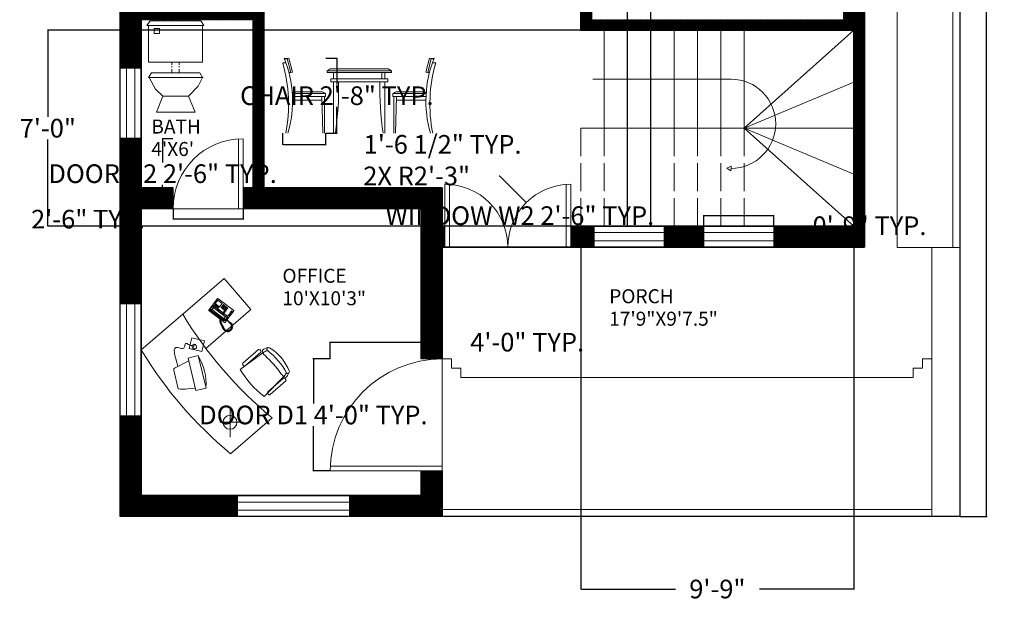
# Model space of a CAD drawing. Units: inches. Extents: x 542 to 1025, y 651 to 1330.
# Tile 1 of 4: x 571 to 993, y 651 to 900. Entities that reach past the tile are written whole.
import ezdxf

# ---------------------------------------------------------------- set-up
doc = ezdxf.new("R2010")
doc.units = ezdxf.units.IN
doc.header["$MEASUREMENT"] = 0
doc.linetypes.add('ACAD_ISO02W100', pattern=[15, 12, -3])
for name, color, linetype, lineweight in [('A-ANNO-DIMS', 2, 'Continuous', 18), ('A-AREA-IDEN', 7, 'Continuous', 18), ('A-DOOR', 3, 'Continuous', 18), ('A-FLOR-EXTR', 7, 'Continuous', 18), ('A-FLOR-FIXT', 9, 'Continuous', 18), ('A-FLOR-STRS', 7, 'Continuous', 18), ('A-FLOR-STRS-HIDN', 8, 'ACAD_ISO02W100', 18), ('A-GLAZ', 4, 'Continuous', 18), ('A-ROOF', 8, 'Continuous', 18), ('A-WALL', 7, 'Continuous', 35), ('A-WALL-PATT', 7, 'Continuous', 13), ('C-PROP', 7, 'Continuous', 25), ('Furniture', 7, 'Continuous', 15)]:
    doc.layers.add(name, color=color, linetype=linetype, lineweight=lineweight)
doc.styles.get("Standard").update_dxf_attribs({"font": 'italic8.shx'})
doc.dimstyles.get("Standard").update_dxf_attribs({"dimtxt": 8, "dimasz": 0.18, "dimexe": 0.18, "dimexo": 0.0625, "dimgap": 0.09, "dimtad": 0, "dimtih": 1, "dimtoh": 1, "dimdec": 4, "dimzin": 0, "dimdsep": 46, "dimlunit": 3, "dimtxsty": 'Standard', "dimcen": 0.09, "dimclrt": 6, "dimadec": 0, "dimazin": 0, "dimtfac": 1, "dimtdec": 4, "dimtofl": 0, "dimtmove": 0, "dimatfit": 3, "dimfxl": 1, "dimtolj": 1, "dimtzin": 0, "dimarcsym": 0})

# ---------------------------------------------------------------- blocks, each defined once
blk = doc.blocks.new('*D4')
at = {"layer": 'A-ANNO-DIMS', "color": 0, "lineweight": -2, "transparency": 16777216}
for p, q in [((974.29, 1287.14), (985.84, 1287.14)), ((985.66, 1286.96), (985.66, 991.99)), ((985.66, 687.32), (985.66, 982.29)), ((974.29, 687.14), (985.84, 687.14))]:
    blk.add_line(p, q, dxfattribs=at)
at = {"layer": 'A-ANNO-DIMS', "color": 0, "transparency": 16777216}
for points in [[(985.63, 1286.96), (985.69, 1286.96), (985.66, 1287.14)], [(985.63, 687.32), (985.69, 687.32), (985.66, 687.14)]]:
    blk.add_solid(points, dxfattribs=at)
at = {"layer": 'Defpoints', "color": 0, "transparency": 16777216}
for p in [(974.23, 1287.14), (974.23, 687.14), (985.66, 687.14)]:
    blk.add_point(p, dxfattribs=at)
at = {"layer": 'A-ANNO-DIMS', "color": 0, "transparency": 16777216, "insert": (985.66, 987.14), "char_height": 8, "attachment_point": 5}
blk.add_mtext("\\A1;50'", dxfattribs=at)
blk = doc.blocks.new('CHAIR-DINING-SIDE')
for p, q in [((1.41, 30.15), (0, 30.15)), ((1.94, 31.92), (2.68, 32.1)), ((1.94, 31.92), (3.43, 26.01)), ((2.7, 32.11), (4.19, 26.2)), ((3.46, 26.01), (4.19, 26.2)), ((18.4, 16.93), (4.13, 16.93)), ((17.12, 17.72), (4.91, 17.72)), ((18.4, 15.75), (18.4, 16.93)), ((18.4, 15.75), (4.19, 15.75)), ((16.86, 14.17), (4.19, 14.17)), ((16.82, 15.75), (17.22, 0)), ((18, 15.75), (18, 0))]:
    blk.add_line(p, q)
for centre, radius, start, end in [((-61.28, 12.41), 63.8, 348.7797, 16.1395), ((1.61, 36.79), 4.8, 258.7985, 282.7633), ((-44.8, 13.77), 49.03, 343.6897, 21.9263), ((1.34, 34.84), 2.99, 258.4671, 281.5329), ((3.04, 27.45), 1.5, 256.0176, 285.0974), ((4.91, 16.93), 0.787, 90, 180), ((17.12, 16.93), 0.787, 0, 90)]:
    blk.add_arc(centre, radius, start, end)
blk = doc.blocks.new('WC-TANK')
for p, q in [((0, 37.14), (1.38, 39.21)), ((1.38, 39.21), (23.19, 39.21)), ((24.51, 37.14), (23.19, 39.21)), ((0, 37.14), (24.51, 37.14)), ((0.71, 37.14), (0.71, 21.45)), ((3.1, 35.95), (3.1, 33.74)), ((5.47, 35.95), (3.1, 35.95)), ((5.47, 33.74), (5.47, 35.95)), ((23.85, 21.45), (23.85, 37.14)), ((3.1, 33.74), (5.47, 33.74)), ((0.71, 21.45), (23.85, 21.45)), ((10.73, 20.35), (10.73, 21.49)), ((12.28, 21.45), (13.82, 21.45)), ((13.82, 21.45), (13.82, 20.35)), ((0.71, 14.94), (1.99, 16.93)), ((1.99, 16.93), (22.71, 16.93)), ((10.73, 19.33), (10.73, 19.84)), ((10.73, 16.85), (10.73, 18.48)), ((13.82, 19.84), (13.82, 19.33)), ((13.82, 18.48), (13.82, 16.85)), ((23.85, 14.94), (22.71, 16.93)), ((0.71, 14.94), (23.85, 14.94)), ((24.1, 14.94), (0.96, 14.94)), ((0.96, 14.94), (3.7, 9.98)), ((13.82, 16.85), (10.73, 16.85)), ((22.02, 11.19), (23.85, 14.94)), ((3.7, 9.98), (6.94, 6.98)), ((17.87, 6.98), (22.02, 11.19)), ((4.14, 0), (6.9, 6.9)), ((17.87, 6.98), (6.94, 6.98)), ((6.94, 6.98), (17.87, 6.98)), ((20.67, 0), (17.91, 6.9)), ((4.14, 0), (20.67, 0)), ((12.4, 0), (4.14, 0))]:
    blk.add_line(p, q)
blk = doc.blocks.new('DOOR-SINGLE-48IN')
for p, q in [((48, 0), (48, 48)), ((0, 0), (48, 0)), ((0.04, 2), (48, 2))]:
    blk.add_line(p, q)
blk.add_arc((48, 0), 48, 90, 180)
blk = doc.blocks.new('DOOR-SINGLE-30IN')
for p, q in [((0, 0), (0, 30)), ((29.93, 2), (0, 2)), ((30, 0), (0, 0))]:
    blk.add_line(p, q)
blk.add_arc((0, 0), 30, 0, 90)
blk = doc.blocks.new('WINDOW-48IN')
for p, q in [((0, 48), (0, 0)), ((9, 48), (0, 48)), ((0, 48), (4.5, 48)), ((2.75, 48), (2.75, 0)), ((6.25, 48), (6.25, 0)), ((9, 0), (9, 48)), ((0, 0), (9, 0))]:
    blk.add_line(p, q)
blk = doc.blocks.new('WINDOW-30IN')
for p, q in [((0, 30), (0, 0)), ((9, 30), (0, 30)), ((0, 30), (4.5, 30)), ((2.75, 30), (2.75, 0)), ((6.25, 30), (6.25, 0)), ((9, 0), (9, 30)), ((0, 0), (9, 0))]:
    blk.add_line(p, q)
blk = doc.blocks.new('*D14')
at = {"layer": 'A-ANNO-DIMS', "color": 0, "lineweight": -2, "transparency": 16777216}
for p, q in [((864.47, 816.14), (864.29, 816.14)), ((864.47, 811.7), (864.47, 816.32)), ((894.29, 816.14), (864.65, 816.14)), ((894.47, 811.7), (894.47, 816.32))]:
    blk.add_line(p, q, dxfattribs=at)
at = {"layer": 'A-ANNO-DIMS', "color": 0, "transparency": 16777216}
for points in [[(864.65, 816.17), (864.65, 816.11), (864.47, 816.14)], [(894.29, 816.17), (894.29, 816.11), (894.47, 816.14)]]:
    blk.add_solid(points, dxfattribs=at)
at = {"layer": 'Defpoints', "color": 0, "transparency": 16777216}
for p in [(864.47, 816.14), (864.47, 811.64), (894.47, 811.64)]:
    blk.add_point(p, dxfattribs=at)
at = {"layer": 'A-ANNO-DIMS', "color": 6, "transparency": 16777216, "insert": (785.54, 816.14), "char_height": 8, "attachment_point": 5}
blk.add_mtext('\\A1;WINDOW W2 2\'-6" TYP.', dxfattribs=at)
blk = doc.blocks.new('*D15')
at = {"layer": 'A-ANNO-DIMS', "color": 0, "lineweight": -2, "transparency": 16777216}
for p, q in [((894.54, 811.64), (899.15, 811.64)), ((898.97, 811.64), (898.97, 811.82)), ((898.97, 811.82), (899.15, 811.82)), ((898.97, 802.82), (898.97, 811.46)), ((894.54, 802.64), (899.15, 802.64))]:
    blk.add_line(p, q, dxfattribs=at)
at = {"layer": 'A-ANNO-DIMS', "color": 0, "transparency": 16777216}
for points in [[(898.94, 811.46), (899, 811.46), (898.97, 811.64)], [(898.94, 802.82), (899, 802.82), (898.97, 802.64)]]:
    blk.add_solid(points, dxfattribs=at)
at = {"layer": 'Defpoints', "color": 0, "transparency": 16777216}
for p in [(894.47, 811.64), (898.97, 811.64), (894.47, 802.64)]:
    blk.add_point(p, dxfattribs=at)
at = {"layer": 'A-ANNO-DIMS', "color": 6, "transparency": 16777216, "insert": (935.43, 811.82), "char_height": 8, "attachment_point": 5}
blk.add_mtext('\\A1;0\'-9" TYP.', dxfattribs=at)
blk = doc.blocks.new('*D16')
at = {"layer": 'A-ANNO-DIMS', "color": 0, "lineweight": -2, "transparency": 16777216}
for p, q in [((704.17, 754.71), (696.85, 754.71)), ((697.03, 754.53), (697.03, 735.56)), ((697.03, 706.89), (697.03, 725.85)), ((704.17, 706.71), (696.85, 706.71))]:
    blk.add_line(p, q, dxfattribs=at)
at = {"layer": 'A-ANNO-DIMS', "color": 0, "transparency": 16777216}
for points in [[(697, 754.53), (697.06, 754.53), (697.03, 754.71)], [(697, 706.89), (697.06, 706.89), (697.03, 706.71)]]:
    blk.add_solid(points, dxfattribs=at)
at = {"layer": 'Defpoints', "color": 0, "transparency": 16777216}
for p in [(697.03, 754.71), (704.23, 754.71), (704.23, 706.71)]:
    blk.add_point(p, dxfattribs=at)
at = {"layer": 'A-ANNO-DIMS', "color": 6, "transparency": 16777216, "insert": (697.03, 730.71), "char_height": 8, "attachment_point": 5}
blk.add_mtext('\\A1;DOOR D1 4\'-0" TYP.', dxfattribs=at)
blk = doc.blocks.new('*D17')
at = {"layer": 'A-ANNO-DIMS', "color": 0, "lineweight": -2, "transparency": 16777216}
for p, q in [((704.23, 754.77), (704.23, 762.09)), ((704.41, 761.91), (752.05, 761.91)), ((752.23, 754.77), (752.23, 762.09)), ((752.23, 761.91), (752.41, 761.91))]:
    blk.add_line(p, q, dxfattribs=at)
at = {"layer": 'A-ANNO-DIMS', "color": 0, "transparency": 16777216}
for points in [[(704.41, 761.94), (704.41, 761.88), (704.23, 761.91)], [(752.05, 761.94), (752.05, 761.88), (752.23, 761.91)]]:
    blk.add_solid(points, dxfattribs=at)
at = {"layer": 'Defpoints', "color": 0, "transparency": 16777216}
for p in [(752.23, 761.91), (704.23, 754.71), (752.23, 754.71)]:
    blk.add_point(p, dxfattribs=at)
at = {"layer": 'A-ANNO-DIMS', "color": 6, "transparency": 16777216, "insert": (788.69, 761.91), "char_height": 8, "attachment_point": 5}
blk.add_mtext('\\A1;4\'-0" TYP.', dxfattribs=at)
blk = doc.blocks.new('*D18')
at = {"layer": 'A-ANNO-DIMS', "color": 0, "lineweight": -2, "transparency": 16777216}
for p, q in [((636.83, 849.14), (632.21, 849.14)), ((632.39, 848.96), (632.39, 838.99)), ((632.39, 819.32), (632.39, 829.29)), ((636.83, 819.14), (632.21, 819.14))]:
    blk.add_line(p, q, dxfattribs=at)
at = {"layer": 'A-ANNO-DIMS', "color": 0, "transparency": 16777216}
for points in [[(632.36, 848.96), (632.42, 848.96), (632.39, 849.14)], [(632.36, 819.32), (632.42, 819.32), (632.39, 819.14)]]:
    blk.add_solid(points, dxfattribs=at)
at = {"layer": 'Defpoints', "color": 0, "transparency": 16777216}
for p in [(632.39, 849.14), (636.89, 849.14), (636.89, 819.14)]:
    blk.add_point(p, dxfattribs=at)
at = {"layer": 'A-ANNO-DIMS', "color": 6, "transparency": 16777216, "insert": (632.39, 834.14), "char_height": 8, "attachment_point": 5}
blk.add_mtext('\\A1;DOOR D2 2\'-6" TYP.', dxfattribs=at)
blk = doc.blocks.new('*D19')
at = {"layer": 'A-ANNO-DIMS', "color": 0, "lineweight": -2, "transparency": 16777216}
for p, q in [((636.89, 819.08), (636.89, 814.46)), ((666.89, 819.08), (666.89, 814.46)), ((636.89, 814.64), (636.71, 814.64)), ((666.71, 814.64), (637.07, 814.64))]:
    blk.add_line(p, q, dxfattribs=at)
at = {"layer": 'A-ANNO-DIMS', "color": 0, "transparency": 16777216}
for points in [[(637.07, 814.67), (637.07, 814.61), (636.89, 814.64)], [(666.71, 814.67), (666.71, 814.61), (666.89, 814.64)]]:
    blk.add_solid(points, dxfattribs=at)
at = {"layer": 'Defpoints', "color": 0, "transparency": 16777216}
for p in [(636.89, 819.14), (666.89, 819.14), (636.89, 814.64)]:
    blk.add_point(p, dxfattribs=at)
at = {"layer": 'A-ANNO-DIMS', "color": 6, "transparency": 16777216, "insert": (600.43, 814.64), "char_height": 8, "attachment_point": 5}
blk.add_mtext('\\A1;2\'-6" TYP.', dxfattribs=at)
blk = doc.blocks.new('*D24')
at = {"layer": 'A-ANNO-DIMS', "color": 0, "lineweight": -2, "transparency": 16777216}
for p, q in [((702.32, 883.63), (707.26, 883.63)), ((707.08, 883.45), (707.08, 872.43)), ((707.08, 851.7), (707.08, 862.72)), ((702.32, 851.52), (707.26, 851.52))]:
    blk.add_line(p, q, dxfattribs=at)
at = {"layer": 'A-ANNO-DIMS', "color": 0, "transparency": 16777216}
for points in [[(707.05, 883.45), (707.11, 883.45), (707.08, 883.63)], [(707.05, 851.7), (707.11, 851.7), (707.08, 851.52)]]:
    blk.add_solid(points, dxfattribs=at)
at = {"layer": 'Defpoints', "color": 0, "transparency": 16777216}
for p in [(702.26, 883.63), (707.08, 883.63), (702.26, 851.52)]:
    blk.add_point(p, dxfattribs=at)
at = {"layer": 'A-ANNO-DIMS', "color": 6, "transparency": 16777216, "insert": (707.08, 867.57), "char_height": 8, "attachment_point": 5}
blk.add_mtext('\\A1;CHAIR 2\'-8" TYP.', dxfattribs=at)
blk = doc.blocks.new('*D25')
at = {"layer": 'A-ANNO-DIMS', "color": 0, "lineweight": -2, "transparency": 16777216}
for p, q in [((683.86, 851.46), (683.86, 846.52)), ((702.26, 851.46), (702.26, 846.52)), ((684.04, 846.7), (702.08, 846.7)), ((702.26, 846.7), (702.44, 846.7))]:
    blk.add_line(p, q, dxfattribs=at)
at = {"layer": 'A-ANNO-DIMS', "color": 0, "transparency": 16777216}
for points in [[(684.04, 846.73), (684.04, 846.67), (683.86, 846.7)], [(702.08, 846.73), (702.08, 846.67), (702.26, 846.7)]]:
    blk.add_solid(points, dxfattribs=at)
at = {"layer": 'Defpoints', "color": 0, "transparency": 16777216}
for p in [(683.86, 851.52), (702.26, 851.52), (702.26, 846.7)]:
    blk.add_point(p, dxfattribs=at)
at = {"layer": 'A-ANNO-DIMS', "color": 6, "transparency": 16777216, "insert": (752.43, 846.7), "char_height": 8, "attachment_point": 5}
blk.add_mtext('\\A1;1\'-6 1/2" TYP.', dxfattribs=at)
blk = doc.blocks.new('*D28')
at = {"layer": 'A-ANNO-DIMS', "color": 0, "lineweight": -2, "transparency": 16777216}
for p, q in [((811.73, 811.58), (811.73, 655.91)), ((928.73, 811.58), (928.73, 655.91)), ((811.91, 656.09), (852.23, 656.09)), ((928.55, 656.09), (888.22, 656.09))]:
    blk.add_line(p, q, dxfattribs=at)
at = {"layer": 'A-ANNO-DIMS', "color": 0, "transparency": 16777216}
for points in [[(811.91, 656.12), (811.91, 656.06), (811.73, 656.09)], [(928.55, 656.12), (928.55, 656.06), (928.73, 656.09)]]:
    blk.add_solid(points, dxfattribs=at)
at = {"layer": 'Defpoints', "color": 0, "transparency": 16777216}
for p in [(811.73, 811.64), (928.73, 811.64), (928.73, 656.09)]:
    blk.add_point(p, dxfattribs=at)
at = {"layer": 'A-ANNO-DIMS', "color": 6, "transparency": 16777216, "insert": (870.23, 656.09), "char_height": 8, "attachment_point": 5}
blk.add_mtext('\\A1;9\'-9"', dxfattribs=at)
blk = doc.blocks.new('*D29')
at = {"layer": 'A-ANNO-DIMS', "color": 0, "lineweight": -2, "transparency": 16777216}
for p, q in [((811.67, 895.64), (583, 895.64)), ((583.18, 895.46), (583.18, 858.49)), ((583.18, 811.82), (583.18, 848.79)), ((811.67, 811.64), (583, 811.64))]:
    blk.add_line(p, q, dxfattribs=at)
at = {"layer": 'A-ANNO-DIMS', "color": 0, "transparency": 16777216}
for points in [[(583.15, 895.46), (583.21, 895.46), (583.18, 895.64)], [(583.15, 811.82), (583.21, 811.82), (583.18, 811.64)]]:
    blk.add_solid(points, dxfattribs=at)
at = {"layer": 'Defpoints', "color": 0, "transparency": 16777216}
for p in [(583.18, 895.64), (811.73, 895.64), (811.73, 811.64)]:
    blk.add_point(p, dxfattribs=at)
at = {"layer": 'A-ANNO-DIMS', "color": 6, "transparency": 16777216, "insert": (583.18, 853.64), "char_height": 8, "attachment_point": 5}
blk.add_mtext('\\A1;7\'-0"', dxfattribs=at)
blk = doc.blocks.new('*D30')
at = {"layer": 'A-ANNO-DIMS', "color": 0, "lineweight": -2, "transparency": 16777216}
for p, q in [((831.73, 811.7), (831.73, 1318.37)), ((831.91, 1318.19), (841.55, 1318.19)), ((841.73, 811.7), (841.73, 1318.37)), ((841.73, 1318.19), (841.91, 1318.19))]:
    blk.add_line(p, q, dxfattribs=at)
at = {"layer": 'A-ANNO-DIMS', "color": 0, "transparency": 16777216}
for points in [[(831.91, 1318.22), (831.91, 1318.16), (831.73, 1318.19)], [(841.55, 1318.22), (841.55, 1318.16), (841.73, 1318.19)]]:
    blk.add_solid(points, dxfattribs=at)
at = {"layer": 'Defpoints', "color": 0, "transparency": 16777216}
for p in [(841.73, 1318.19), (831.73, 811.64), (841.73, 811.64)]:
    blk.add_point(p, dxfattribs=at)
at = {"layer": 'A-ANNO-DIMS', "color": 6, "transparency": 16777216, "insert": (862.57, 1318.19), "char_height": 8, "attachment_point": 5}
blk.add_mtext('\\A1;0\'-10"', dxfattribs=at)
blk = doc.blocks.new('*D36')
at = {"layer": 'A-ANNO-DIMS', "color": 0, "lineweight": -2, "transparency": 16777216}
for p, q in [((776.64, 833.19), (776.82, 833.19)), ((776.82, 833.19), (788.15, 821.86)), ((807.27, 802.64), (807.45, 802.64)), ((807.36, 802.55), (807.36, 802.73))]:
    blk.add_line(p, q, dxfattribs=at)
at = {"layer": 'A-ANNO-DIMS', "color": 0, "transparency": 16777216}
blk.add_solid([(788.17, 821.88), (788.12, 821.84), (788.27, 821.73)], dxfattribs=at)
at = {"layer": 'Defpoints', "color": 0, "transparency": 16777216}
for p in [(788.27, 821.73), (807.36, 802.64)]:
    blk.add_point(p, dxfattribs=at)
at = {"layer": 'A-ANNO-DIMS', "color": 6, "transparency": 16777216, "insert": (741.31, 833.19), "char_height": 8, "attachment_point": 5}
blk.add_mtext('\\A1;2X R2\'-3"', dxfattribs=at)

msp = doc.modelspace()

# ---------------------------------------------------------------- hatches: boundary and pattern name
at = {"layer": 'A-WALL-PATT'}
h = msp.add_hatch(dxfattribs=at)
h.set_pattern_fill('ANSI31', color=256)
h.set_pattern_definition([(45, (-552.11989, -271.07657), (-0.088388348, 0.088388348), [])])
h.paths.add_polyline_path([(715.041, 1218.14134), (623.2294, 1218.14134), (623.2294, 1278.14134), (687.2294, 1278.14134), (687.2294, 1287.14134), (614.2294, 1287.14134), (614.2294, 1150.81788), (618.7294, 1150.81788), (623.2294, 1150.81788), (623.2294, 1209.14134), (715.041, 1209.14134)])
h.paths.add_polyline_path([(864.47291, 1213.64134), (864.47291, 1218.14134), (763.041, 1218.14134), (763.041, 1213.64134), (763.041, 1209.14134), (776.2294, 1209.14134), (776.2294, 1065.14134), (769.45548, 1065.14134), (769.45548, 1060.64134), (776.2294, 1060.64134), (776.2294, 1053.42968), (780.7294, 1053.42968), (780.7294, 1144.64134), (780.7294, 1209.14134), (840.2294, 1209.14134), (840.2294, 1181.73273), (844.7294, 1181.73273), (844.7294, 1209.14134), (864.47291, 1209.14134)])
h.paths.add_polyline_path([(933.2294, 1218.14134), (894.47291, 1218.14134), (894.47291, 1209.14134), (924.2294, 1209.14134), (924.2294, 1144.64134), (924.2294, 1100.56821), (928.7294, 1100.56821), (933.2294, 1100.56821)])
h.paths.add_polyline_path([(933.2294, 1052.56821), (924.2294, 1052.56821), (924.2294, 1000.64134), (780.7294, 1000.64134), (780.7294, 1005.42968), (776.2294, 1005.42968), (776.2294, 996.14134), (780.7294, 996.14134), (811.7294, 996.14134), (811.7294, 987.24818), (816.2294, 987.24818), (816.2294, 996.14134), (924.2294, 996.14134), (924.2294, 975.07641), (928.7294, 975.07641), (933.2294, 975.07641)])
h.paths.add_polyline_path([(924.2294, 1149.14134), (844.7294, 1149.14134), (844.7294, 1151.73273), (840.2294, 1151.73273), (840.2294, 1149.14134), (831.41283, 1149.14134), (831.41283, 1144.64134), (924.2294, 1144.64134)])
h.paths.add_polyline_path([(623.2294, 1102.81788), (614.2294, 1102.81788), (614.2294, 1047.96339), (618.7294, 1047.96339), (623.2294, 1047.96339), (623.2294, 1060.64134), (655.18423, 1060.64134), (655.18423, 1065.14134), (623.2294, 1065.14134)])
h.paths.add_polyline_path([(721.45548, 1065.14134), (685.18423, 1065.14134), (685.18423, 1060.64134), (695.2294, 1060.64134), (695.2294, 1000.64134), (623.2294, 1000.64134), (623.2294, 1017.96339), (614.2294, 1017.96339), (614.2294, 996.14134), (666.7294, 996.14134), (666.7294, 976.55402), (671.2294, 976.55402), (675.7294, 976.55402), (675.7294, 996.14134), (699.7294, 996.14134), (699.7294, 1060.64134), (721.45548, 1060.64134)])
h.paths.add_polyline_path([(675.7294, 928.55402), (666.7294, 928.55402), (666.7294, 904.64134), (614.2294, 904.64134), (614.2294, 879.38817), (618.7294, 879.38817), (623.2294, 879.38817), (623.2294, 900.14134), (671.2294, 900.14134), (671.2294, 828.14134), (666.89138, 828.14134), (666.89138, 819.14134), (743.2294, 819.14134), (743.2294, 754.70501), (752.2294, 754.70501), (752.2294, 802.64134), (753.36467, 802.64134), (753.36467, 811.64134), (752.2294, 811.64134), (752.2294, 828.14134), (675.7294, 828.14134)])
h.paths.add_polyline_path([(636.89138, 828.14134), (623.2294, 828.14134), (623.2294, 849.38817), (614.2294, 849.38817), (614.2294, 778.30684), (618.7294, 778.30684), (623.2294, 778.30684), (623.2294, 819.14134), (636.89138, 819.14134)], flags=17)
h.paths.add_polyline_path([(864.47291, 811.64134), (847.39014, 811.64134), (847.39014, 802.64134), (864.47291, 802.64134)], flags=17)
h.paths.add_polyline_path([(817.39014, 811.64134), (807.36467, 811.64134), (807.36467, 802.64134), (817.39014, 802.64134), (817.39014, 807.14134)])
h.paths.add_polyline_path([(933.2294, 927.07641), (924.2294, 927.07641), (924.2294, 900.14134), (816.2294, 900.14134), (816.2294, 951.24818), (811.7294, 951.24818), (811.7294, 895.64134), (928.7294, 895.64134), (928.7294, 811.64134), (894.47291, 811.64134), (894.47291, 802.64134), (933.2294, 802.64134)])
h.paths.add_polyline_path([(752.2294, 706.70501), (743.2294, 706.70501), (743.2294, 696.14134), (712.47774, 696.14134), (712.47774, 691.64134), (712.47774, 687.14134), (752.2294, 687.14134)])
h.paths.add_polyline_path([(664.47774, 696.14134), (623.2294, 696.14134), (623.2294, 730.30684), (614.2294, 730.30684), (614.2294, 687.14134), (664.47774, 687.14134)])
h.paths.add_polyline_path([(925.1985, 1143.73295), (966.26993, 1143.73295), (966.26993, 1152.66152), (925.1985, 1152.66152)], flags=9)
h.paths.add_polyline_path([(925.4366, 1152.0031), (965.31755, 1152.0031), (965.31755, 1159.5031), (925.4366, 1159.5031)], flags=9)

# ---------------------------------------------------------------- linework, layer by layer
at = {"layer": 'A-DOOR'}
for p, q in [((636.89138, 819.14134), (636.89138, 828.14134)), ((666.89138, 819.14134), (666.89138, 828.14134)), ((753.36467, 802.64134), (753.36467, 829.64134)), ((755.36467, 802.64134), (755.36467, 829.56716)), ((805.36467, 802.64134), (805.36467, 829.56716)), ((807.36467, 802.64134), (807.36467, 829.64134)), ((753.36467, 811.64134), (753.36467, 802.64134)), ((807.36467, 811.64134), (807.36467, 802.64134)), ((753.36467, 802.64134), (780.36467, 802.64134)), ((805.36467, 802.64134), (807.36467, 802.64134)), ((752.2294, 754.70501), (743.2294, 754.70501)), ((752.2294, 706.70501), (743.2294, 706.70501))]:
    msp.add_line(p, q, dxfattribs=at)
for centre, start, end in [((753.36467, 802.64134), 0, 90), ((807.36467, 802.64134), 90, 180)]:
    msp.add_arc(centre, 27, start, end, dxfattribs=at)
at = {"layer": 'A-FLOR-EXTR'}
for p, q in [((971.2294, 1284.14134), (971.2294, 802.5643)), ((974.2294, 802.5643), (947.2294, 802.5643)), ((962.2294, 802.5643), (962.2294, 687.14134)), ((752.2294, 754.70501), (756.2294, 754.70501)), ((756.2294, 754.70501), (756.2294, 750.70501)), ((958.2294, 754.70501), (962.2294, 754.70501)), ((958.2294, 754.70501), (958.2294, 750.70501)), ((756.2294, 750.70501), (760.2294, 750.70501)), ((760.2294, 750.70501), (760.2294, 746.70501)), ((958.2294, 750.70501), (954.2294, 750.70501)), ((954.2294, 750.70501), (954.2294, 746.70501)), ((760.2294, 746.70501), (954.2294, 746.70501)), ((962.2294, 690.14134), (752.2294, 690.14134))]:
    msp.add_line(p, q, dxfattribs=at)
at = {"layer": 'A-FLOR-STRS'}
for p, q in [((821.7294, 853.64134), (821.7294, 895.64134)), ((831.7294, 853.64134), (831.7294, 895.64134)), ((841.7294, 853.64134), (841.7294, 895.64134)), ((851.7294, 853.64134), (851.7294, 895.64134)), ((861.7294, 853.64134), (861.7294, 895.64134)), ((871.7294, 853.64134), (871.7294, 895.64134)), ((881.7294, 853.64134), (881.7294, 895.64134)), ((881.7294, 853.64134), (928.7294, 895.64134)), ((816.86539, 874.64134), (876.09796, 874.64134)), ((881.7294, 853.64134), (928.7294, 873.37034)), ((928.7294, 853.64134), (811.7294, 853.64134)), ((881.7294, 853.64134), (928.7294, 811.64134)), ((881.7294, 853.64134), (928.7294, 833.99499)), ((876.09796, 837.41066), (874.31702, 836.49381)), ((876.00479, 835.41501), (874.31702, 836.49381)), ((876.09796, 836.41066), (876.00479, 835.41501)), ((876.09796, 836.41066), (876.09796, 837.41066))]:
    msp.add_line(p, q, dxfattribs=at)
msp.add_arc((876.09796, 855.526), 19.11534, 270, 90, dxfattribs=at)
at = {"layer": 'A-FLOR-STRS-HIDN'}
for p, q in [((811.7294, 853.64134), (811.7294, 811.64134)), ((821.7294, 853.64134), (821.7294, 811.64134)), ((831.7294, 853.64134), (831.7294, 811.64134)), ((841.7294, 853.64134), (841.7294, 811.64134)), ((851.7294, 853.64134), (851.7294, 811.64134)), ((861.7294, 853.64134), (861.7294, 811.64134)), ((871.7294, 853.64134), (871.7294, 811.64134)), ((881.7294, 853.64134), (881.7294, 811.64134))]:
    msp.add_line(p, q, dxfattribs=at)
at = {"layer": 'A-ROOF'}
msp.add_line((947.2294, 1236.14134), (947.2294, 802.5643), dxfattribs=at)
at = {"layer": 'A-WALL'}
for p, q in [((933.2294, 1218.14134), (933.2294, 802.64134)), ((675.7294, 828.14134), (675.7294, 996.14134)), ((811.7294, 951.24818), (811.7294, 895.64134)), ((816.2294, 951.24818), (816.2294, 900.14134)), ((623.2294, 828.14134), (623.2294, 900.14134)), ((671.2294, 828.14134), (671.2294, 900.14134)), ((811.7294, 895.64134), (928.7294, 895.64134)), ((928.7294, 895.64134), (928.7294, 811.64134)), ((623.2294, 828.14134), (636.89138, 828.14134)), ((666.89138, 828.14134), (671.2294, 828.14134)), ((675.7294, 828.14134), (752.2294, 828.14134)), ((752.2294, 811.64134), (752.2294, 828.14134)), ((623.2294, 696.14134), (623.2294, 819.14134)), ((623.2294, 819.14134), (636.89138, 819.14134)), ((666.89138, 819.14134), (743.2294, 819.14134)), ((743.2294, 754.70501), (743.2294, 819.14134)), ((752.2294, 811.64134), (753.36467, 811.64134)), ((807.36467, 811.64134), (928.7294, 811.64134)), ((752.2294, 802.64134), (933.2294, 802.64134)), ((752.2294, 754.70501), (752.2294, 802.64134)), ((743.2294, 696.14134), (743.2294, 706.70501)), ((752.2294, 687.14134), (752.2294, 706.70501)), ((743.2294, 696.14134), (623.2294, 696.14134))]:
    msp.add_line(p, q, dxfattribs=at)
at = {"layer": 'C-PROP'}
for p, q in [((614.2294, 687.14134), (614.2294, 1287.14134)), ((974.2294, 1287.14134), (974.2294, 687.14134)), ((974.2294, 687.14134), (614.2294, 687.14134))]:
    msp.add_line(p, q, dxfattribs=at)
at = {"layer": 'Furniture'}
for p, q in [((702.89755, 878.29037), (704.2755, 879.07777)), ((702.89755, 878.29037), (730.45655, 878.29037)), ((702.89755, 878.29037), (702.89755, 877.50297)), ((704.2755, 879.07777), (729.0786, 879.07777)), ((729.0786, 879.07777), (730.45655, 878.29037)), ((730.45655, 878.29037), (730.45655, 877.50297)), ((702.89755, 877.50297), (730.45655, 877.50297)), ((704.47235, 874.74707), (728.88175, 874.74707)), ((704.47235, 874.74707), (704.47235, 873.56597)), ((705.65345, 877.50297), (705.65345, 874.74707)), ((707.02104, 874.74707), (707.02104, 877.50297)), ((726.33306, 874.74707), (726.33306, 877.50297)), ((727.70065, 877.50297), (727.70065, 874.74707)), ((728.88175, 874.74707), (728.88175, 873.56597)), ((704.47235, 873.56597), (728.88175, 873.56597)), ((705.65345, 873.56597), (705.65345, 851.51877)), ((727.70065, 873.56597), (727.70065, 851.51877)), ((641.00668, 773.89231, -13.39871), (658.78395, 789.21706, -13.39871)), ((658.78395, 789.21706, -13.39871), (670.27751, 775.8841, -13.39871)), ((655.92529, 780.61826), (652.16955, 775.69536)), ((653.85709, 777.60108), (652.73037, 776.12421)), ((653.75609, 777.36661), (652.85472, 776.18511)), ((653.75609, 777.36661), (654.00478, 777.48841)), ((654.20828, 776.63222), (653.75609, 777.36661)), ((654.25347, 777.61021), (653.85709, 777.60108)), ((654.00478, 777.48841), (654.23925, 777.38741)), ((654.23925, 777.38741), (655.56844, 776.37336)), ((654.23925, 777.38741), (654.3443, 776.60633)), ((660.21017, 773.06577), (654.25347, 777.61021)), ((654.66406, 777.84214), (654.96451, 778.23597)), ((654.81174, 777.72947), (654.66406, 777.84214)), ((655.1122, 778.1233), (654.81174, 777.72947)), ((654.95943, 777.6168), (655.25989, 778.01063)), ((655.10712, 777.50412), (654.95943, 777.6168)), ((654.96451, 778.23597), (655.1122, 778.1233)), ((656.06789, 779.88641), (654.97873, 778.45877)), ((654.97873, 778.45877), (656.8002, 777.06915)), ((655.40758, 777.89796), (655.10712, 777.50412)), ((655.2548, 777.39145), (655.55526, 777.78528)), ((655.40249, 777.27878), (655.2548, 777.39145)), ((655.25989, 778.01063), (655.40758, 777.89796)), ((655.70295, 777.67261), (655.40249, 777.27878)), ((655.55018, 777.16611), (655.85064, 777.55994)), ((655.69786, 777.05344), (655.55018, 777.16611)), ((655.55526, 777.78528), (655.70295, 777.67261)), ((655.99832, 777.44727), (655.69786, 777.05344)), ((655.84555, 776.94076), (656.14601, 777.3346)), ((655.99324, 776.82809), (655.84555, 776.94076)), ((655.85064, 777.55994), (655.99832, 777.44727)), ((656.09886, 780.64161), (655.92529, 780.61826)), ((656.2937, 777.22192), (655.99324, 776.82809)), ((657.88937, 778.49679), (656.06789, 779.88641)), ((662.89246, 775.45869), (656.09886, 780.64161)), ((656.14093, 776.71542), (656.44138, 777.10925)), ((656.28861, 776.60275), (656.14093, 776.71542)), ((656.14601, 777.3346), (656.2937, 777.22192)), ((656.58907, 776.99658), (656.28861, 776.60275)), ((656.44138, 777.10925), (656.58907, 776.99658)), ((656.8002, 777.06915), (657.88937, 778.49679)), ((657.69141, 777.01229), (657.46606, 776.71692)), ((657.46606, 776.71692), (657.76144, 776.49158)), ((657.98678, 776.78695), (657.69141, 777.01229)), ((657.76144, 776.49158), (657.98678, 776.78695)), ((658.06698, 777.50458), (657.84164, 777.20921)), ((657.84164, 777.20921), (658.13701, 776.98387)), ((658.36236, 777.27924), (658.06698, 777.50458)), ((658.13701, 776.98387), (658.36236, 777.27924)), ((658.44256, 777.99687), (658.21721, 777.7015)), ((658.21721, 777.7015), (658.51259, 777.47616)), ((658.6085, 777.09145), (658.38316, 776.79608)), ((658.38316, 776.79608), (658.67853, 776.57074)), ((658.73793, 777.77153), (658.44256, 777.99687)), ((658.51259, 777.47616), (658.73793, 777.77153)), ((658.90387, 776.86611), (658.6085, 777.09145)), ((658.67853, 776.57074), (658.90387, 776.86611)), ((658.98407, 777.58374), (658.75873, 777.28837)), ((658.75873, 777.28837), (659.0541, 777.06302)), ((659.15002, 776.67832), (658.92468, 776.38295)), ((659.27945, 777.3584), (658.98407, 777.58374)), ((659.0541, 777.06302), (659.27945, 777.3584)), ((659.44539, 776.45298), (659.15002, 776.67832)), ((659.52559, 777.17061), (659.30025, 776.87524)), ((659.30025, 776.87524), (659.59562, 776.64989)), ((659.82097, 776.94527), (659.52559, 777.17061)), ((659.59562, 776.64989), (659.82097, 776.94527)), ((660.06711, 776.75748), (659.84177, 776.46211)), ((660.36249, 776.53214), (660.06711, 776.75748)), ((623.2294, 758.56757, -13.39871), (641.00668, 773.89231, -13.39871)), ((670.27751, 775.8841, -13.39871), (650.93231, 759.20774, -13.39871)), ((652.16955, 775.69536), (652.1929, 775.52179)), ((652.1929, 775.52179), (658.9865, 770.33887)), ((652.73037, 776.12421), (652.78873, 775.69028)), ((652.78873, 775.69028), (658.69621, 771.18339)), ((652.85472, 776.18511), (652.80294, 775.91308)), ((652.80294, 775.91308), (652.9623, 775.71362)), ((653.68248, 775.94301), (652.85472, 776.18511)), ((652.9623, 775.71362), (653.74338, 775.81867)), ((652.9623, 775.71362), (654.29148, 774.69957)), ((653.68248, 775.94301), (654.20828, 776.63222)), ((653.74338, 775.81867), (653.68248, 775.94301)), ((655.95868, 774.12859), (653.74338, 775.81867)), ((654.3443, 776.60633), (654.20828, 776.63222)), ((654.29148, 774.69957), (654.61274, 774.61024)), ((656.5596, 774.91625), (654.3443, 776.60633)), ((654.61274, 774.61024), (654.97156, 774.57014)), ((654.97156, 774.57014), (655.35372, 774.35647)), ((655.35372, 774.35647), (655.84601, 773.9809)), ((655.56844, 776.37336), (655.73947, 776.08711)), ((655.73947, 776.08711), (655.87294, 775.75164)), ((656.78136, 773.26731), (655.84601, 773.9809)), ((655.87294, 775.75164), (656.17998, 775.43951)), ((655.95868, 774.12859), (658.61705, 772.10049)), ((656.17998, 775.43951), (656.67227, 775.06394)), ((656.5596, 774.91625), (659.21797, 772.88815)), ((657.60762, 774.35035), (656.67227, 775.06394)), ((657.08841, 772.95518), (656.78136, 773.26731)), ((657.22188, 772.6197), (657.08841, 772.95518)), ((657.39291, 772.33346), (657.22188, 772.6197)), ((657.98978, 774.13667), (657.60762, 774.35035)), ((658.3486, 774.09657), (657.98978, 774.13667)), ((658.23293, 776.59916), (658.00758, 776.30379)), ((658.00758, 776.30379), (658.30296, 776.07845)), ((658.5283, 776.37382), (658.23293, 776.59916)), ((658.30296, 776.07845), (658.5283, 776.37382)), ((658.66986, 774.00724), (658.3486, 774.09657)), ((658.77445, 776.18603), (658.5491, 775.89066)), ((658.5491, 775.89066), (658.84448, 775.66531)), ((658.86528, 775.18215), (658.56482, 774.78832)), ((658.56482, 774.78832), (658.86019, 774.56298)), ((659.99904, 772.9932), (658.66986, 774.00724)), ((658.75306, 772.0746), (659.27887, 772.76381)), ((659.06982, 775.96069), (658.77445, 776.18603)), ((658.84448, 775.66531), (659.06982, 775.96069)), ((658.86019, 774.56298), (659.16065, 774.95681)), ((659.16065, 774.95681), (658.86528, 775.18215)), ((658.92468, 776.38295), (659.22005, 776.1576)), ((659.31596, 775.7729), (659.09062, 775.47753)), ((659.09062, 775.47753), (659.38599, 775.25218)), ((659.99904, 772.9932), (659.21797, 772.88815)), ((659.21797, 772.88815), (659.27887, 772.76381)), ((659.22005, 776.1576), (659.44539, 776.45298)), ((659.27887, 772.76381), (660.10663, 772.52171)), ((659.61134, 775.54756), (659.31596, 775.7729)), ((659.38599, 775.25218), (659.61134, 775.54756)), ((659.69154, 776.26519), (659.46619, 775.96982)), ((659.46619, 775.96982), (659.76157, 775.74447)), ((659.98691, 776.03985), (659.69154, 776.26519)), ((660.10663, 772.52171), (659.69167, 771.97779)), ((659.74029, 771.93944), (660.26853, 772.63184)), ((659.76157, 775.74447), (659.98691, 776.03985)), ((659.84177, 776.46211), (660.13714, 776.23676)), ((660.1584, 772.79374), (659.99904, 772.9932)), ((660.1009, 771.59542), (662.91581, 775.28512)), ((660.10663, 772.52171), (660.1584, 772.79374)), ((660.13714, 776.23676), (660.36249, 776.53214)), ((660.26853, 772.63184), (660.21017, 773.06577)), ((660.47308, 773.41037), (660.84865, 773.90266)), ((660.76845, 773.18503), (660.47308, 773.41037)), ((661.14402, 773.67732), (660.76845, 773.18503)), ((660.84865, 773.90266), (661.14402, 773.67732)), ((660.99888, 774.09958), (661.37445, 774.59187)), ((661.29425, 773.87423), (660.99888, 774.09958)), ((661.66983, 774.36652), (661.29425, 773.87423)), ((661.37445, 774.59187), (661.66983, 774.36652)), ((661.52468, 774.78878), (661.90026, 775.28107)), ((661.82006, 774.56344), (661.52468, 774.78878)), ((662.19563, 775.05573), (661.82006, 774.56344)), ((661.90026, 775.28107), (662.19563, 775.05573)), ((662.91581, 775.28512), (662.89246, 775.45869)), ((656.86741, 770.65787), (656.92111, 770.79028)), ((656.94667, 770.53437), (656.86741, 770.65787)), ((656.92111, 770.79028), (657.04796, 770.97721)), ((657.32747, 770.49603), (656.94667, 770.53437)), ((656.96496, 771.26119), (656.98638, 771.43398)), ((657.04796, 770.97721), (656.96496, 771.26119)), ((656.98638, 771.43398), (657.16502, 771.7285)), ((657.0501, 770.29784), (657.32747, 770.49603)), ((657.13883, 770.10406), (657.0501, 770.29784)), ((657.54954, 770.04291), (657.13883, 770.10406)), ((657.21556, 770.92816), (657.13955, 770.82853)), ((657.13955, 770.82853), (657.33045, 770.87203)), ((657.21043, 771.23153), (657.20135, 771.03356)), ((657.20135, 771.03356), (657.21556, 770.92816)), ((657.21429, 771.40196), (657.21043, 771.23153)), ((657.31271, 771.61582), (657.21429, 771.40196)), ((657.2394, 769.82244), (657.54954, 770.04291)), ((657.3381, 769.62105), (657.2394, 769.82244)), ((657.33045, 770.87203), (657.4927, 770.46454)), ((657.72699, 769.65534), (657.3381, 769.62105)), ((658.72209, 771.31941), (657.39291, 772.33346)), ((657.40215, 769.47762), (657.72699, 769.65534)), ((657.54546, 769.21067), (657.40215, 769.47762)), ((657.4927, 770.46454), (657.7878, 769.73504)), ((657.91155, 769.21508), (657.54546, 769.21067)), ((657.61662, 769.01453), (657.91155, 769.21508)), ((657.74236, 768.74523), (657.61662, 769.01453)), ((658.12553, 768.68933), (657.74236, 768.74523)), ((657.7878, 769.73504), (658.03691, 769.21401)), ((657.83296, 768.47121), (658.12553, 768.68933)), ((657.90885, 768.23994), (657.83296, 768.47121)), ((658.33476, 768.19871), (657.90885, 768.23994)), ((658.03691, 769.21401), (658.00364, 769.12906)), ((658.00364, 769.12906), (658.1062, 769.0981)), ((658.1062, 769.0981), (658.44117, 768.33819)), ((658.44117, 768.33819), (659.12742, 767.29452)), ((658.72209, 771.31941), (658.61705, 772.10049)), ((658.61705, 772.10049), (658.75306, 772.0746)), ((658.69621, 771.18339), (659.17937, 771.2042)), ((658.95657, 771.21841), (658.72209, 771.31941)), ((658.75306, 772.0746), (659.20525, 771.34021)), ((659.20525, 771.34021), (658.95657, 771.21841)), ((658.9865, 770.33887), (659.16007, 770.36222)), ((659.16007, 770.36222), (659.96939, 771.42305)), ((659.17937, 771.2042), (659.61918, 771.78069)), ((659.57267, 771.82181), (659.20525, 771.34021)), ((659.43314, 771.94517), (659.54581, 772.09286)), ((659.80598, 771.61554), (659.43314, 771.94517)), ((659.54581, 772.09286), (659.9651, 771.76209)), ((660.07178, 771.30243), (659.80598, 771.61554)), ((659.9651, 771.76209), (660.37234, 771.26227)), ((660.44911, 770.82543), (660.07178, 771.30243)), ((660.37234, 771.26227), (660.74967, 770.78527)), ((660.66556, 770.61301), (660.44911, 770.82543)), ((660.93235, 770.42523), (660.66556, 770.61301)), ((660.74967, 770.78527), (661.01646, 770.59749)), ((660.92514, 770.14704), (660.93235, 770.42523)), ((661.18482, 770.01196), (660.92514, 770.14704)), ((661.01646, 770.59749), (661.05347, 770.52197)), ((661.05347, 770.52197), (661.24673, 770.5479)), ((661.77486, 769.48301), (661.18482, 770.01196)), ((661.24673, 770.5479), (661.50119, 770.3853)), ((661.50119, 770.3853), (661.33061, 770.05835)), ((661.33061, 770.05835), (661.7129, 770.20802)), ((661.7129, 770.20802), (661.96686, 769.98274)), ((661.96686, 769.98274), (661.75355, 769.64112)), ((661.75355, 769.64112), (662.18568, 769.75276)), ((661.96454, 768.73937), (661.77486, 769.48301)), ((661.84084, 767.9984), (661.96454, 768.73937)), ((662.40978, 768.28937), (662.02799, 768.20237)), ((662.31615, 769.44832), (662.02832, 769.19507)), ((662.02832, 769.19507), (662.41386, 769.1216)), ((662.47929, 768.83527), (662.135, 768.73542)), ((662.135, 768.73542), (662.43457, 768.56992)), ((662.18568, 769.75276), (662.31615, 769.44832)), ((662.43457, 768.56992), (662.40978, 768.28937)), ((662.41386, 769.1216), (662.47929, 768.83527)), ((658.07684, 767.92265), (658.33476, 768.19871)), ((658.3075, 767.60482), (658.07684, 767.92265)), ((658.63757, 767.81008), (658.3075, 767.60482)), ((658.38438, 767.49888), (658.63757, 767.81008)), ((658.56046, 767.25422), (658.38438, 767.49888)), ((658.91945, 767.31133), (658.56046, 767.25422)), ((658.71424, 767.04234), (658.91945, 767.31133)), ((658.92545, 766.80239), (658.71424, 767.04234)), ((659.25079, 767.04278), (658.92545, 766.80239)), ((659.12742, 767.29452), (659.9815, 766.86359)), ((659.20271, 766.66967), (659.25079, 767.04278)), ((659.43249, 766.55742), (659.20271, 766.66967)), ((659.65814, 766.87386), (659.43249, 766.55742)), ((659.74489, 766.42941), (659.65814, 766.87386)), ((660.00507, 766.35701), (659.74489, 766.42941)), ((659.9815, 766.86359), (660.74459, 766.97492)), ((660.13577, 766.71437), (660.00507, 766.35701)), ((660.29852, 766.36955), (660.13577, 766.71437)), ((660.51695, 766.4078), (660.29852, 766.36955)), ((660.61014, 766.77802), (660.51695, 766.4078)), ((660.78809, 766.45312), (660.61014, 766.77802)), ((660.74459, 766.97492), (661.43464, 767.36262)), ((661.04927, 766.50605), (660.78809, 766.45312)), ((661.22596, 766.65496), (660.94969, 766.91301)), ((660.94969, 766.91301), (661.04927, 766.50605)), ((661.42732, 766.75352), (661.22596, 766.65496)), ((661.40275, 767.13477), (661.42732, 766.75352)), ((661.67951, 766.93938), (661.40275, 767.13477)), ((661.43464, 767.36262), (661.84084, 767.9984)), ((661.98067, 767.29279), (661.63837, 767.44361)), ((661.63837, 767.44361), (661.87377, 767.09065)), ((661.87377, 767.09065), (661.67951, 766.93938)), ((662.27996, 767.72643), (661.912, 767.80226)), ((661.912, 767.80226), (662.08995, 767.47737)), ((662.08995, 767.47737), (661.98067, 767.29279)), ((662.02799, 768.20237), (662.37976, 767.98128)), ((662.37976, 767.98128), (662.27996, 767.72643)), ((643.83961, 759.26943), (644.96815, 763.78997)), ((644.96815, 763.78997), (650.33086, 762.45119)), ((645.12066, 760.45566), (645.72909, 760.15188)), ((646.16006, 761.0126), (645.39952, 759.36711)), ((650.33086, 762.45119), (649.20232, 757.93065)), ((647.65904, 756.15701), (643.32219, 755.11125)), ((649.20232, 757.93065), (643.83961, 759.26943)), ((651.02395, 742.20779), (647.65904, 756.15701)), ((675.42637, 757.279), (665.61177, 750.26403)), ((673.5017, 758.71022), (666.79366, 752.85004)), ((667.76132, 751.74238), (674.46937, 757.60256)), ((674.51333, 758.25431), (674.15346, 758.66625)), ((643.61079, 753.91672), (637.44215, 750.75838)), ((643.32219, 755.11125), (646.6871, 741.16203)), ((666.74969, 752.19829), (667.10957, 751.78635)), ((637.14381, 749.98369), (639.09154, 741.90018)), ((675.90044, 738.65121), (684.21734, 747.07649)), ((684.2367, 746.42206), (677.52866, 740.56188)), ((678.49632, 739.45422), (685.20437, 745.3144)), ((685.24833, 745.96615), (684.88846, 746.37809)), ((646.44796, 742.24736), (643.21929, 741.84767)), ((646.6871, 741.16203), (651.02395, 742.20779)), ((677.48469, 739.91013), (677.84457, 739.49819)), ((661.2873, 733.6755), (661.28743, 721.18)), ((656.96793, 727.57646), (667.09626, 727.57657)), ((679.31854, 729.44912, -13.39871), (661.54126, 714.12437, -13.39871))]:
    msp.add_line(p, q, dxfattribs=at)
msp.add_circle((661.28737, 727.57651), 2.98107, dxfattribs=at)
for centre, radius, start, end in [((575.66651, 870.69673), 132.17307, 351.6570855, 1.2438872), ((857.68758, 870.69673), 132.17307, 178.7561128, 188.3429145), ((791.653, 865.02085, -13.39871), 176.06454, 211.1704614, 230.3549234), ((773.87572, 849.6961, -13.39871), 176.06454, 211.1704614, 230.3549234), ((629.72417, 744.45068), 21.27464, 355.1004131, 32.021149), ((673.8056, 758.36236), 0.46191, 41.1406281, 131.1406281), ((674.16547, 757.95042), 0.46191, 311.1406281, 41.1406281), ((677.53347, 758.09785), 2.28192, 171.6547996, 239.0366044), ((678.02206, 755.91106), 3.72594, 93.9380812, 137.4840012), ((678.87863, 753.55889), 5.03083, 107.6314706, 133.3999796), ((640.85288, 718.00876), 52.10367, 35.7526888, 47.0421676), ((677.75073, 758.92595), 0.68628, 57.8202444, 231.6150969), ((656.86006, 732.5542), 32.95728, 29.4212771, 51.6150969), ((667.57825, 742.01658), 20.52308, 20.9291574, 58.5688421), ((667.09756, 752.50218), 0.46191, 131.1406281, 221.1406281), ((667.45743, 752.09024), 0.46191, 221.1406281, 311.1406281), ((637.85352, 750.15516), 0.73014, 124.2922666, 193.5825686), ((700.373, 770.69747), 40.32206, 210.4479789, 232.6323545), ((689.80261, 753.25101), 8.21293, 215.7526888, 229.2550437), ((679.30044, 751.77928), 6.81266, 317.0446482, 335.1138685), ((684.97703, 747.64966), 0.8196, 229.2550437, 321.9234576), ((686.03011, 749.0766), 0.57043, 215.7013467, 2.0615592), ((676.36436, 753.26004), 11.09556, 326.5507798, 339.353274), ((684.5406, 746.0742), 0.46191, 41.1406281, 131.1406281), ((684.90047, 745.66226), 0.46191, 311.1406281, 41.1406281), ((641.36387, 758.26167), 16.51853, 262.0931916, 276.4492789), ((677.83256, 740.21402), 0.46191, 131.1406281, 221.1406281), ((678.19243, 739.80208), 0.46191, 221.1406281, 311.1406281)]:
    msp.add_arc(centre, radius, start, end, dxfattribs=at)
msp.add_open_spline([(638.97543, 751.54342), (637.60655, 755.88887), (635.7854, 761.66999), (642.00851, 758.27197), (641.76159, 762.80218), (644.65118, 759.4982), (646.12682, 761.75558), (647.72757, 759.10095), (645.05559, 758.89547), (645.08216, 760.04055), (645.09531, 760.60755)], degree=3, knots=[0, 0, 0, 0, 8.15293561, 10.846566517, 12.870898549, 15.828178785, 16.932193764, 18.800108591, 20.265071851, 21.701967483, 21.701967483, 21.701967483, 21.701967483], dxfattribs=at)

# ---------------------------------------------------------------- block references
at = {"layer": 'A-DOOR', "rotation": 90.00000000000006}
msp.add_blockref('DOOR-SINGLE-30IN', (666.89111, 819.14094), dxfattribs=at)
at = {"layer": 'A-DOOR'}
msp.add_blockref('DOOR-SINGLE-48IN', (704.229, 706.705), dxfattribs=at)
at = {"layer": 'A-FLOR-FIXT'}
msp.add_blockref('WC-TANK', (625.61519, 860.44867), dxfattribs=at)
at = {"layer": 'A-GLAZ'}
for name, p in [('WINDOW-30IN', (614.229, 849.388)), ('WINDOW-48IN', (614.229, 730.30663))]:
    msp.add_blockref(name, p, dxfattribs=at)
for name, p, rotation in [('WINDOW-30IN', (847.39031, 802.64094), 89.99999999999969), ('WINDOW-30IN', (894.47308, 802.64094), 89.9999999999994), ('WINDOW-48IN', (664.47753, 696.14174), 270.0000000000001)]:
    msp.add_blockref(name, p, dxfattribs=dict(at, rotation=rotation))
at = {"layer": 'Furniture'}
msp.add_blockref('CHAIR-DINING-SIDE', (683.863, 851.519), dxfattribs=at)
at = {"layer": 'Furniture', "extrusion": (0, 0, -1), "zscale": -1}
msp.add_blockref('CHAIR-DINING-SIDE', (-749.49109, 851.519), dxfattribs=at)

# ---------------------------------------------------------------- texts
at = {"layer": 'A-AREA-IDEN'}
for s, p in [('BATH', (627.56513, 851.35127)), ("4'X6'", (627.56513, 841.71279)), ('OFFICE', (683.75409, 787.38012)), ('10\'X10\'3"', (683.75409, 777.74165)), ('PORCH', (823.85401, 778.60111)), ('17\'9"X9\'7.5"', (823.85401, 768.96264))]:
    msp.add_text(s, height=6, dxfattribs=at).set_placement(p)

# ---------------------------------------------------------------- dimensions: what is measured, and where the dimension line sits
at = {"layer": 'A-ANNO-DIMS'}
for base, p1, p2, picture, middle in [((841.7294, 1318.19134), (831.7294, 811.64134), (841.7294, 811.64134), '*D30', (862.57083, 1318.19134)), ((928.7294, 656.09134), (811.7294, 811.64134), (928.7294, 811.64134), '*D28', (870.2294, 656.09134))]:
    dim = msp.add_linear_dim(base=base, p1=p1, p2=p2, dimstyle='Standard', override={"dimdec": 1, "dimlfac": 1, "dimrnd": 0, "dimzin": 1, "dimdsep": 46, "dimlunit": 4, "dimfrac": 2}, dxfattribs=at)
    dim.commit()
    dim.dimension.update_dxf_attribs({"geometry": picture, "text_midpoint": middle})
for base, p1, p2, override, picture, middle in [((985.65631, 687.14134), (974.2294, 1287.14134), (974.2294, 687.14134), {"dimclrd": 0, "dimclre": 0, "dimclrt": 0}, '*D4', (985.65631, 987.14134)), ((583.1794, 895.64134), (811.7294, 811.64134), (811.7294, 895.64134), {"dimdec": 1, "dimlfac": 1, "dimrnd": 0, "dimzin": 1, "dimdsep": 46, "dimlunit": 4, "dimfrac": 2}, '*D29', (583.1794, 853.64134))]:
    dim = msp.add_linear_dim(base=base, p1=p1, p2=p2, angle=90, dimstyle='Standard', override=override, dxfattribs=at)
    dim.commit()
    dim.dimension.update_dxf_attribs({"geometry": picture, "text_midpoint": middle})
for base, p1, p2, angle, text, picture, middle in [((707.07641, 883.62826), (702.25998, 851.51877), (702.25998, 883.62826), 90, 'CHAIR <> TYP.', '*D24', (707.07641, 867.57351)), ((632.39138, 849.14134), (636.89138, 819.14134), (636.89138, 849.14134), 90, 'DOOR D2 <> TYP.', '*D18', (632.39138, 834.14134)), ((864.47291, 816.14134), (894.47291, 811.64134), (864.47291, 811.64134), 180, 'WINDOW W2 <> TYP.', '*D14', (785.53625, 816.14134)), ((636.89138, 814.64134), (666.89138, 819.14134), (636.89138, 819.14134), 180, '<> TYP.', '*D19', (600.4309, 814.64134)), ((898.97291, 811.64134), (894.47291, 802.64134), (894.47291, 811.64134), 90, '<> TYP.', '*D15', (935.43339, 811.82134)), ((697.0294, 754.70501), (704.2294, 706.70501), (704.2294, 754.70501), 90, 'DOOR D1 <> TYP.', '*D16', (697.0294, 730.70501))]:
    dim = msp.add_linear_dim(base=base, p1=p1, p2=p2, angle=angle, text=text, dimstyle='Standard', override={"dimdec": 1, "dimlfac": 1, "dimrnd": 0, "dimzin": 1, "dimdsep": 46, "dimlunit": 4, "dimfrac": 2}, dxfattribs=at)
    dim.commit()
    dim.dimension.update_dxf_attribs({"geometry": picture, "text_midpoint": middle})
for base, p1, p2, picture, middle in [((702.25998, 846.70235), (683.86295, 851.51877), (702.25998, 851.51877), '*D25', (752.43475, 846.70235)), ((752.2294, 761.90501), (704.2294, 754.70501), (752.2294, 754.70501), '*D17', (788.68988, 761.90501))]:
    dim = msp.add_linear_dim(base=base, p1=p1, p2=p2, text='<> TYP.', dimstyle='Standard', override={"dimdec": 1, "dimlfac": 1, "dimrnd": 0, "dimzin": 1, "dimdsep": 46, "dimlunit": 4, "dimfrac": 2}, dxfattribs=at)
    dim.commit()
    dim.dimension.update_dxf_attribs({"geometry": picture, "text_midpoint": middle})
dim = msp.add_radius_dim(center=(807.36467, 802.64134), mpoint=(788.27278, 821.73322), text='2X <>', dimstyle='Standard', override={"dimdec": 1, "dimlfac": 1, "dimrnd": 0, "dimzin": 1, "dimdsep": 46, "dimlunit": 4, "dimfrac": 2}, dxfattribs=at)
dim.commit()
dim.dimension.update_dxf_attribs({"geometry": '*D36', "text_midpoint": (741.30956, 833.18834), "dimtype": 164})

doc.saveas('drawing.dxf')
